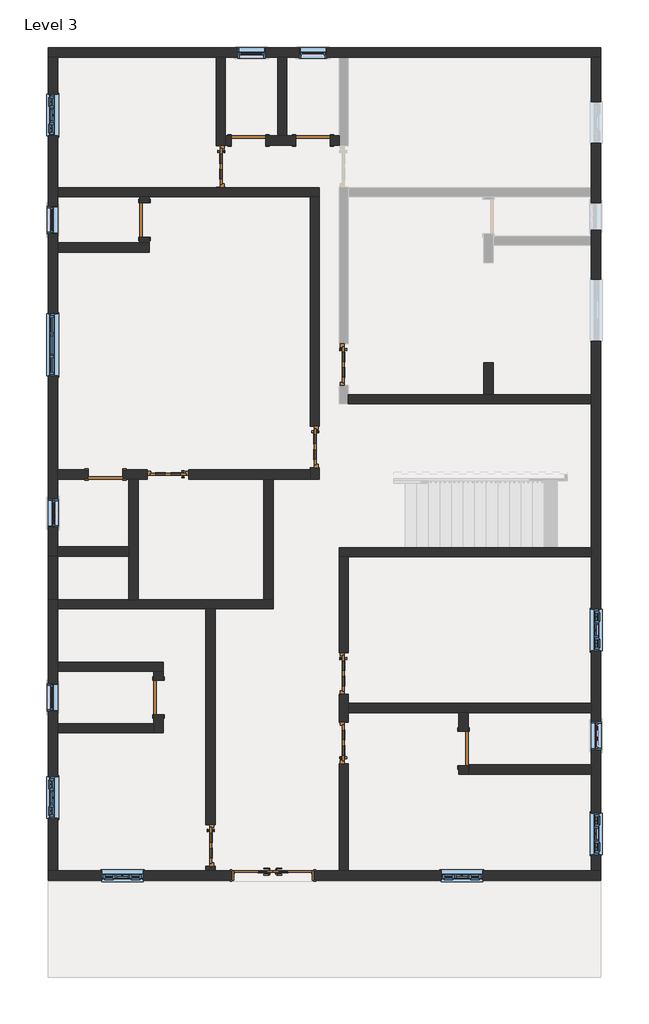
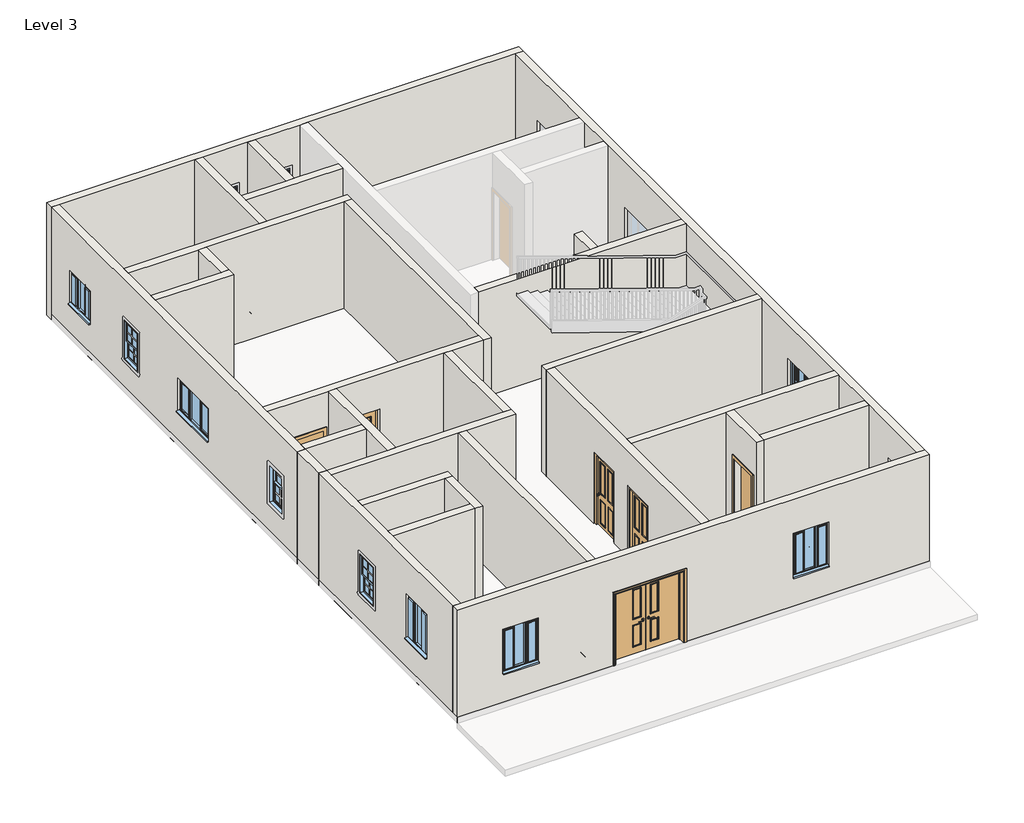
# One storey, part 1 of 3: 29 walls, 14 doors, 13 windows.
# Revit data of these elements (continued)
# Type "Windows_Tpl_w-Glazing_Cross-Bars : 910x1210mm"
#   Type Mark = "25"
#   Operation = "TriplePanelVertical"
#   Construction Type Id = "GSP4R"
#   Manufacturer = "Revit"
#   Keynote = "L10"
#   Analytic Construction = "1/8 in Pilkington single glazing"
#   Wrap Layers (Ext) from Ext = 0' - 4.03543"
#   Wrap Layers (Int) from Ext = 0' - 6.98819"
#   Window Board Projection = 0' - 0.98425"
#   Window Board Extension = 0' - 0.98425"
#   Visual Light Transmittance = 0.9
#   Solar Heat Gain Coefficient = 0.78
#   Rough Width = 2' - 11.82677"
#   Rough Height = 3' - 11.6378"
#   Height = 3' - 11.6378"
#   Width = 2' - 11.82677"
#   Heat Transfer Coefficient (U) = 0.6496 BTU/(h·ft²·°F)
#   Glazing Thickness = 0' - 0.94488"
#   Glazing Bar Thickness = 0' - 0.7874"
#   FrameOffset - External = 0' - 1.9685"
#   Frame Depth = 0' - 2.55906"
#   Default Head Height = 6' - 11.07087"
#   Cill Depth = 0' - 3.44488"
#   Cavity Closer Width = 0' - 1.9685"
#   Cavity Closer Offset from Ext = 0' - 4.03543"
#   Cavity Closer Depth = 0' - 3.34646"
#   Vis - Glazing Bars = yes
#   Vis - Cavity Closers = yes
#   Define Thermal Properties by = 1
#   Material Trim = Window Frame
#   Material Glazing Bars = Window Frame
#   Material Glass = Glass
#   Material Frame = Window Frame
#   Wall Closure = (empty or 0)
# Type "Windows_Tpl_w-Glazing_Cross-Bars : 910x910mm"
#   Type Mark = "24"
#   Operation = "TriplePanelVertical"
#   Construction Type Id = "GSP4R"
#   Manufacturer = "Revit"
#   Keynote = "L10"
#   Analytic Construction = "1/8 in Pilkington single glazing"
#   Wrap Layers (Ext) from Ext = 0' - 4.03543"
#   Wrap Layers (Int) from Ext = 0' - 6.98819"
#   Window Board Projection = 0' - 0.98425"
#   Window Board Extension = 0' - 0.98425"
#   Visual Light Transmittance = 0.9
#   Solar Heat Gain Coefficient = 0.78
#   Rough Width = 2' - 11.82677"
#   Rough Height = 2' - 11.82677"
#   Height = 2' - 11.82677"
#   Width = 2' - 11.82677"
#   Heat Transfer Coefficient (U) = 0.6496 BTU/(h·ft²·°F)
#   Glazing Thickness = 0' - 0.94488"
#   Glazing Bar Thickness = 0' - 0.7874"
#   FrameOffset - External = 0' - 1.9685"
#   Frame Depth = 0' - 2.55906"
#   Default Head Height = 6' - 11.07087"
#   Cill Depth = 0' - 3.44488"
#   Cavity Closer Width = 0' - 1.9685"
#   Cavity Closer Offset from Ext = 0' - 4.03543"
#   Cavity Closer Depth = 0' - 3.34646"
#   Vis - Glazing Bars = yes
#   Vis - Cavity Closers = yes
#   Define Thermal Properties by = 1
#   Material Trim = Window Frame
#   Material Glazing Bars = Window Frame
#   Material Glass = Glass
#   Material Frame = Window Frame
#   Wall Closure = (empty or 0)
# Elements 1, 2, 3, 4, 5, 6, 7 (IfcDoor, "Doors_ExtSgl_2 : 2'x7\"")
#   Phase Created = New Construction
#   Materials on its faces: "Door - Panel", "Door - Handle", "Door - Frame/Mullion", "Door - Glazing"
# Element 8 (IfcDoor, "Doors_IntDbl_3 : 1810x2110mm")
#   Phase Created = New Construction
#   Materials on its faces: "Door - Panel", "Door - Handle", "Door - Architrave", "Door - Frame/Mullion", "Door - Glazing"
# Elements 9, 10, 11, 12, 13, 14 (IfcDoor, "Single-Flush : 30\" x 80\"")
#   Phase Created = New Construction
#   Materials on its faces: "Door - Frame", "Door - Panel"
# Elements 15, 16, 17, 18, 19, 20, 21, 22, 23, 24, 25, 26, 27, 28, 29, 30, 31, 32, 33, 34, 35, 36, 37 (IfcWall, "Generic - 4.5\" p")
#   Top Offset = 0' - 0"
#   Base Offset = 0' - 0"
#   Unconnected Height = 10' - 0"
#   wall height = 10' - 0"
#   Phase Created = New Construction
#   Base Constraint = Level 3
#   Materials on its faces: "Default Wall"
# Element 38 (IfcWall, "Generic - 4.5\" p")
#   Top Offset = 0' - 0"
#   Base Offset = 0' - 0"
#   Unconnected Height = 10' - 0"
#   wall height = 10' - 0"
#   Phase Created = New Construction
#   Base Constraint = Level 3
#   Materials on its faces: "Default Wall", "Door - Panel"
# Elements 39, 41, 42, 43 (IfcWall, "Generic - 9\" w")
#   Top Offset = 0' - 0"
#   Base Offset = 0' - 0"
#   Unconnected Height = 10' - 0"
#   wall height = 10' - 0"
#   Phase Created = New Construction
#   Base Constraint = Level 3
#   Materials on its faces: "Default Wall", "Door - Panel"
# Element 40 (IfcWall, "Generic - 9\" w")
#   Top Offset = 0' - 0"
#   Base Offset = 0' - 0"
#   Unconnected Height = 10' - 0"
#   wall height = 10' - 0"
#   Phase Created = New Construction
#   Base Constraint = Level 3
#   Materials on its faces: "Default Wall", "Door - Panel", "Default Mass Interior Wall"
# Element 44 (IfcWindow, "Window-Double-Hung : 24\" x 42\"")
#   Mark = "26"
#   Window Inset = 0' - 0"
#   Interior Wall Closure = 0' - 1 1/2"
#   Frame Extension = 0' - 1 1/4"
#   Exterior Wall Closure = 0' - 0 1/2"
#   Interior Trim Visibility = yes
#   Indicator Visibility = yes
#   Exterior Trim Visibility = yes
#   Phase Created = New Construction
#   Materials on its faces: "Wood - Stained", "Glass", "Clad - White"
# Element 45 (IfcWindow, "Window-Double-Hung : 24\" x 42\"")
#   Mark = "27"
#   Window Inset = 0' - 0"
#   Interior Wall Closure = 0' - 1 1/2"
#   Frame Extension = 0' - 1 1/4"
#   Exterior Wall Closure = 0' - 0 1/2"
#   Interior Trim Visibility = yes
#   Indicator Visibility = yes
#   Exterior Trim Visibility = yes
#   Phase Created = New Construction
#   Materials on its faces: "Wood - Stained", "Glass", "Clad - White"
# Element 46 (IfcWindow, "Window-Double-Hung : 24\" x 42\"")
#   Mark = "28"
#   Window Inset = 0' - 0"
#   Interior Wall Closure = 0' - 1 1/2"
#   Frame Extension = 0' - 1 1/4"
#   Exterior Wall Closure = 0' - 0 1/2"
#   Interior Trim Visibility = yes
#   Indicator Visibility = yes
#   Exterior Trim Visibility = yes
#   Phase Created = New Construction
#   Materials on its faces: "Wood - Stained", "Glass", "Clad - White"
# Element 47 (IfcWindow, "Window-Double-Hung : 24\" x 42\"")
#   Mark = "30"
#   Window Inset = 0' - 0"
#   Interior Wall Closure = 0' - 1 1/2"
#   Frame Extension = 0' - 1 1/4"
#   Exterior Wall Closure = 0' - 0 1/2"
#   Interior Trim Visibility = yes
#   Indicator Visibility = yes
#   Exterior Trim Visibility = yes
#   Phase Created = New Construction
#   Materials on its faces: "Wood - Stained", "Glass", "Clad - White"
# Element 48 (IfcWindow, "Window-Double-Hung : 24\" x 42\"")
#   Mark = "31"
#   Window Inset = 0' - 0"
#   Interior Wall Closure = 0' - 1 1/2"
#   Frame Extension = 0' - 1 1/4"
#   Exterior Wall Closure = 0' - 0 1/2"
#   Interior Trim Visibility = yes
#   Indicator Visibility = yes
#   Exterior Trim Visibility = yes
#   Phase Created = New Construction
#   Materials on its faces: "Wood - Stained", "Glass", "Clad - White"
# Element 49 (IfcWindow, "Window-Double-Hung : 24\" x 42\"")
#   Mark = "32"
#   Window Inset = 0' - 0"
#   Interior Wall Closure = 0' - 1 1/2"
#   Frame Extension = 0' - 1 1/4"
#   Exterior Wall Closure = 0' - 0 1/2"
#   Interior Trim Visibility = yes
#   Indicator Visibility = yes
#   Exterior Trim Visibility = yes
#   Phase Created = New Construction
#   Materials on its faces: "Wood - Stained", "Glass", "Clad - White"
# Element 50 (IfcWindow, "Windows_Tpl_Plain : 1360x910mm")
#   Mark = "23"
#   Phase Created = New Construction
#   Materials on its faces: "Window Frame", "Glass"
# Element 51 (IfcWindow, "Windows_Tpl_w-Glazing_Cross-Bars : 910x1210mm")
#   Mark = "17"
#   Phase Created = New Construction
#   Materials on its faces: "Window Frame", "Glass"
# Element 52 (IfcWindow, "Windows_Tpl_w-Glazing_Cross-Bars : 910x1210mm")
#   Mark = "18"
#   Phase Created = New Construction
#   Materials on its faces: "Window Frame", "Glass"
# Element 53 (IfcWindow, "Windows_Tpl_w-Glazing_Cross-Bars : 910x1210mm")
#   Mark = "19"
#   Phase Created = New Construction
#   Materials on its faces: "Window Frame", "Glass"
# Element 54 (IfcWindow, "Windows_Tpl_w-Glazing_Cross-Bars : 910x1210mm")
#   Mark = "20"
#   Phase Created = New Construction
#   Materials on its faces: "Window Frame", "Glass"
# Element 55 (IfcWindow, "Windows_Tpl_w-Glazing_Cross-Bars : 910x1210mm")
#   Mark = "21"
#   Phase Created = New Construction
#   Materials on its faces: "Window Frame", "Glass"
# Element 56 (IfcWindow, "Windows_Tpl_w-Glazing_Cross-Bars : 910x910mm")
#   Mark = "24"
#   Phase Created = New Construction
#   Materials on its faces: "Window Frame", "Glass"
# Materials
#   "Door - Glazing": colour RGB 0 0 255, transparency 0.75
#   "Door - Panel": class "Wood", colour RGB 210 159 95, transparency 0, Cost = 0
#   "Door - Frame/Mullion": class "Wood", colour RGB 212 179 113, transparency 0
#   "Door - Handle": colour RGB 246 240 166, transparency 0
#   "Door - Architrave": class "Wood", colour RGB 154 90 5, transparency 0
#   "Door - Frame": colour RGB 118 70 51, transparency 0, Cost = 0
#   "Wood - Stained": class "Wood", colour RGB 224 178 126, transparency 0, Cost = 0
#   "Clad - White": class "Wood", colour RGB 242 242 238, transparency 0, Cost = 0
#   "Glass": class "Glass", colour RGB 0 128 192, transparency 0.75, Description = "Soda Lime Glass", Cost = 0
#   "Window Frame": colour RGB 249 249 249, transparency 0
#   "Default Wall": colour RGB 128 128 128, transparency 0, Cost = 0
#   "Default Mass Interior Wall": class "Generic", colour RGB 195 229 126, transparency 0, Cost = 0
